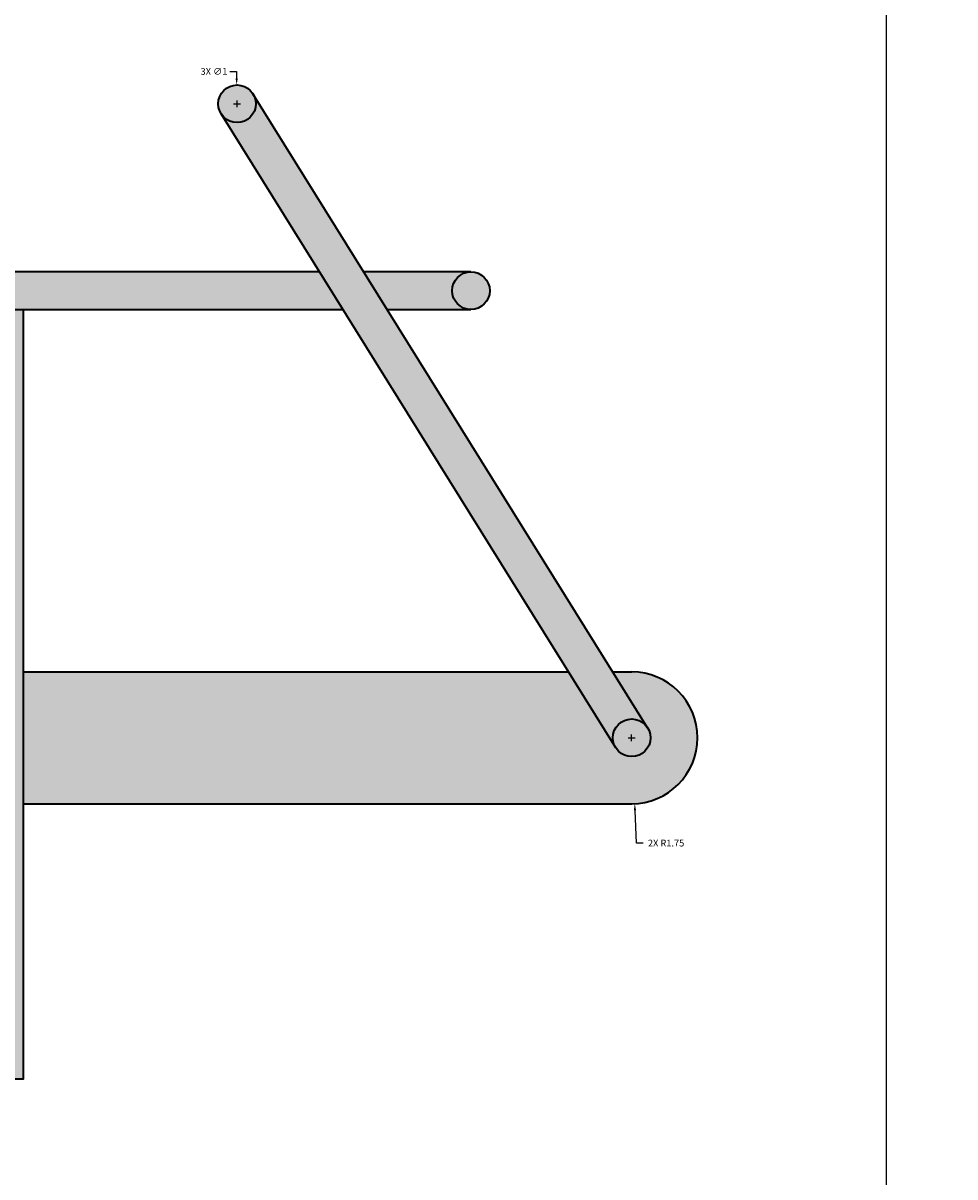
# Model space of a CAD drawing. Units: millimetres. Extents: x -11 to 280, y -4 to 208.
# Tile 54 of 55: x 237 to 262, y 142 to 173. Entities that reach past the tile are written whole.
import ezdxf

# ---------------------------------------------------------------- set-up
doc = ezdxf.new("R2010")
doc.units = ezdxf.units.MM
for name, color, linetype, lineweight in [('M-DIMS', 2, 'Continuous', 18), ('M-HYDR-EQPM', 7, 'Continuous', 35), ('M-HYDR-EQPM-PATT', 252, 'Continuous', 13)]:
    doc.layers.add(name, color=color, linetype=linetype, lineweight=lineweight)
doc.layers.add('M-HYDR-SUCT-PATT', color=221, linetype='Continuous', lineweight=13, true_color=0xff7fdf)
doc.styles.get("Standard").update_dxf_attribs({"font": 'arial.ttf'})
doc.dimstyles.get("Standard").update_dxf_attribs({"dimtxt": 0.18, "dimasz": 0.18, "dimexe": 0.18, "dimexo": 0.0625, "dimgap": 0.09, "dimtad": 0, "dimtih": 1, "dimtoh": 1, "dimdec": 4, "dimzin": 0, "dimdsep": 46, "dimtxsty": 'Standard', "dimcen": 0.09, "dimadec": 0, "dimazin": 0, "dimtfac": 1, "dimtdec": 4, "dimtofl": 0, "dimtmove": 0, "dimatfit": 3, "dimfxl": 1, "dimtolj": 1, "dimtzin": 0, "dimarcsym": 0})

# ---------------------------------------------------------------- blocks, each defined once
blk = doc.blocks.new('*D5')
at = {"layer": 'Defpoints', "color": 0, "transparency": 16777216}
for p in [(24.759, 192.645), (-10.087, 11.435), (261.686, 11.435)]:
    blk.add_point(p, dxfattribs=at)
at = {"layer": 'M-DIMS', "color": 0, "lineweight": -2, "transparency": 16777216}
for p, q in [((24.696, 192.645), (-10.267, 192.645)), ((-10.087, 192.465), (-10.087, 102.222)), ((-10.087, 11.615), (-10.087, 101.858)), ((261.624, 11.435), (-10.267, 11.435))]:
    blk.add_line(p, q, dxfattribs=at)
at = {"layer": 'M-DIMS', "color": 0, "transparency": 16777216}
for points in [[(-10.117, 192.465), (-10.057, 192.465), (-10.087, 192.645)], [(-10.117, 11.615), (-10.057, 11.615), (-10.087, 11.435)]]:
    blk.add_solid(points, dxfattribs=at)
at = {"layer": 'M-DIMS', "color": 0, "transparency": 16777216, "insert": (-10.087, 102.04), "char_height": 0.18, "attachment_point": 5}
blk.add_mtext('\\A1;181.2', dxfattribs=at)
blk = doc.blocks.new('*D22')
at = {"layer": 'Defpoints', "color": 0, "transparency": 16777216}
for p in [(259.871, 207.495), (231.68, 34.723), (259.871, 34.723)]:
    blk.add_point(p, dxfattribs=at)
at = {"layer": 'M-DIMS', "color": 0, "lineweight": -2, "transparency": 16777216}
for p, q in [((231.68, 34.785), (231.68, 207.675)), ((231.86, 207.495), (245.38, 207.495)), ((259.691, 207.495), (246.171, 207.495)), ((259.871, 34.785), (259.871, 207.675))]:
    blk.add_line(p, q, dxfattribs=at)
at = {"layer": 'M-DIMS', "color": 0, "transparency": 16777216}
for points in [[(231.86, 207.525), (231.86, 207.465), (231.68, 207.495)], [(259.691, 207.525), (259.691, 207.465), (259.871, 207.495)]]:
    blk.add_solid(points, dxfattribs=at)
at = {"layer": 'M-DIMS', "color": 0, "transparency": 16777216, "insert": (245.776, 207.495), "char_height": 0.18, "attachment_point": 5}
blk.add_mtext('\\A1;28.19', dxfattribs=at)
blk = doc.blocks.new('*D33')
at = {"layer": 'Defpoints', "color": 0, "transparency": 16777216}
for p in [(242.61, 171.067), (242.625, 170.067)]:
    blk.add_point(p, dxfattribs=at)
at = {"layer": 'M-DIMS', "color": 0, "lineweight": -2, "transparency": 16777216}
for p, q in [((242.425, 171.427), (242.605, 171.427)), ((242.605, 171.427), (242.608, 171.247)), ((242.528, 170.567), (242.708, 170.567)), ((242.618, 170.477), (242.618, 170.657))]:
    blk.add_line(p, q, dxfattribs=at)
at = {"layer": 'M-DIMS', "color": 0, "transparency": 16777216}
blk.add_solid([(242.638, 171.247), (242.578, 171.246), (242.61, 171.067)], dxfattribs=at)
at = {"layer": 'M-DIMS', "color": 0, "transparency": 16777216, "insert": (242.007, 171.427), "char_height": 0.18, "attachment_point": 5}
blk.add_mtext('\\A1;3X ∅1', dxfattribs=at)
blk = doc.blocks.new('*D34')
at = {"layer": 'Defpoints', "color": 0, "transparency": 16777216}
for p in [(253.1, 153.727), (253.181, 151.979)]:
    blk.add_point(p, dxfattribs=at)
at = {"layer": 'M-DIMS', "color": 0, "lineweight": -2, "transparency": 16777216}
for p, q in [((253.01, 153.727), (253.19, 153.727)), ((253.1, 153.637), (253.1, 153.817)), ((253.229, 150.93), (253.189, 151.799)), ((253.409, 150.93), (253.229, 150.93))]:
    blk.add_line(p, q, dxfattribs=at)
at = {"layer": 'M-DIMS', "color": 0, "transparency": 16777216}
blk.add_solid([(253.219, 151.8), (253.159, 151.797), (253.181, 151.979)], dxfattribs=at)
at = {"layer": 'M-DIMS', "color": 0, "transparency": 16777216, "insert": (254.015, 150.93), "char_height": 0.18, "attachment_point": 5}
blk.add_mtext('\\A1;2X R1.75', dxfattribs=at)

msp = doc.modelspace()

# ---------------------------------------------------------------- hatches: boundary and pattern name
at = {"layer": 'M-HYDR-EQPM-PATT'}
h = msp.add_hatch(color=256, dxfattribs=at)
h.set_gradient(color1=(0, 255, 255), color2=(34, 52, 110), tint=1, name='INVCYLINDER')
h.paths.add_polyline_path([(243.0423, 170.8308, -0.1401047), (243.1178, 170.5666, -0.7542249), (242.1933, 170.3024), (252.676, 153.4626, -0.1401047), (252.6005, 153.7268, -0.7542249), (253.5249, 153.991)])
h.paths.add_polyline_path([(243.1178, 170.5666, 0.1401047), (243.0423, 170.8308, 0.7542249), (242.1178, 170.5666, 1)])
h.paths.add_polyline_path([(252.6005, 153.7268, 0.1401047), (252.676, 153.4626, 0.7542249), (253.6005, 153.7268, 1)])
h = msp.add_hatch(color=256, dxfattribs=at)
h.set_gradient(color1=(248, 153, 30), color2=(248, 153, 30), tint=1)
h.paths.add_polyline_path([(236.9353, 165.103), (205.5315, 165.103), (205.5315, 144.6609), (236.9353, 144.6609)])
h.paths.add_polyline_path([(244.8074, 166.103), (205.5315, 166.103), (205.5315, 165.103), (236.9353, 165.103), (245.4299, 165.103)])
h.paths.add_polyline_path([(248.3313, 165.603, -0.4142136), (248.8313, 166.103), (245.9853, 166.103), (246.6078, 165.103), (248.8313, 165.103, -0.4142136)])
h.paths.add_polyline_path([(249.3313, 165.603, 1), (248.3313, 165.603, 0.4142136), (248.8313, 165.103, 0.4142136)])
at = {"layer": 'M-HYDR-SUCT-PATT'}
h = msp.add_hatch(color=256, dxfattribs=at)
h.set_gradient(color1=(255, 127, 223), color2=(255, 127, 223), tint=1, name='INVCYLINDER')
h.paths.add_polyline_path([(91.3629, 155.4768), (91.3629, 132.4768), (58.3629, 132.4768), (58.3629, 153.9768), (54.8629, 153.9768), (54.8629, 128.9768), (94.8629, 128.9768), (94.8629, 151.9768), (205.5315, 151.9768), (205.5315, 155.4768)])
h.paths.add_polyline_path([(91.3, 114.9452, 1), (78.8273, 114.9452), (78.8273, 108.8141), (42.6453, 108.8141), (42.6453, 153.9768), (39.1453, 153.9768), (39.1453, 105.3141), (78.8273, 105.3141), (78.8273, 98.1491, 1), (91.3, 98.1491), (91.3, 105.3141), (95.5776, 105.3141), (95.5776, 108.8141), (91.3, 108.8141)])
h.paths.add_polyline_path([(228.7, 138.4081), (232.2, 138.4081), (232.2, 144.6609), (228.7, 144.6609)])
h.paths.add_polyline_path([(253.1005, 151.9768, 1), (253.1005, 155.4768), (252.6001, 155.4768), (253.5249, 153.991, -0.1401047), (253.6005, 153.7268, -0.7542249), (252.676, 153.4626), (251.4221, 155.4768), (236.9353, 155.4768), (236.9353, 151.9768)])
h.paths.add_polyline_path([(30.8182, 40.7626), (30.8182, 36.7626), (60.8182, 36.7626), (60.8182, 40.7626)])

# ---------------------------------------------------------------- linework, layer by layer
at = {"layer": 'M-HYDR-EQPM'}
for p, q in [((253.5249, 153.991), (243.0423, 170.8308)), ((252.676, 153.4626), (242.1933, 170.3024)), ((244.8074, 166.103), (205.5315, 166.103)), ((248.8313, 166.103), (245.9853, 166.103)), ((236.9353, 165.103), (245.4299, 165.103)), ((246.6078, 165.103), (248.8313, 165.103))]:
    msp.add_line(p, q, dxfattribs=at)
msp.add_lwpolyline([(205.5315, 165.103), (236.9353, 165.103), (236.9353, 144.6609), (205.5315, 144.6609)], close=True, dxfattribs=at)
for points in [[(236.9353, 155.4768), (251.4221, 155.4768)], [(252.6001, 155.4768), (253.1005, 155.4768)], [(236.9353, 151.9768), (253.1005, 151.9768)]]:
    msp.add_lwpolyline(points, dxfattribs=at)
for centre in [(242.6178, 170.5666), (248.8313, 165.603), (253.1005, 153.7268)]:
    msp.add_circle(centre, 0.5, dxfattribs=at)
msp.add_arc((253.1005, 153.7268), 1.75, 270, 90, dxfattribs=at)

# ---------------------------------------------------------------- dimensions: what is measured, and where the dimension line sits
at = {"layer": 'M-DIMS'}
dim = msp.add_linear_dim(base=(259.871, 207.495), p1=(231.6803, 34.7226), p2=(259.871, 34.7226), dimstyle='Standard', override={"dimdec": 2, "dimlfac": 1, "dimrnd": 0, "dimzin": 0, "dimdsep": 46, "dimlunit": 2}, dxfattribs=at)
dim.commit()
dim.dimension.update_dxf_attribs({"geometry": '*D22', "text_midpoint": (245.7757, 207.495)})
dim = msp.add_linear_dim(base=(-10.0865, 11.4346), p1=(24.7588, 192.645), p2=(261.6863, 11.4346), angle=90, dimstyle='Standard', override={"dimdec": 1, "dimlfac": 1, "dimrnd": 0, "dimzin": 0, "dimdsep": 46, "dimlunit": 2}, dxfattribs=at)
dim.commit()
dim.dimension.update_dxf_attribs({"geometry": '*D5', "text_midpoint": (-10.0865, 102.0398)})
dim = msp.add_diameter_dim_2p(p1=(242.6251, 170.0666), p2=(242.6105, 171.0665), text='3X <>', dimstyle='Standard', override={"dimdec": 0, "dimlfac": 1, "dimrnd": 0, "dimzin": 0, "dimdsep": 46, "dimlunit": 2}, dxfattribs=at)
dim.commit()
dim.dimension.update_dxf_attribs({"geometry": '*D33', "text_midpoint": (242.0071, 171.4265), "dimtype": 163})
dim = msp.add_radius_dim(center=(253.1005, 153.7268), mpoint=(253.181, 151.9787), text='2X <>', dimstyle='Standard', override={"dimdec": 2, "dimlfac": 1, "dimrnd": 0, "dimzin": 0, "dimdsep": 46, "dimlunit": 2}, dxfattribs=at)
dim.commit()
dim.dimension.update_dxf_attribs({"geometry": '*D34', "text_midpoint": (254.0148, 150.9298), "dimtype": 164})

doc.saveas('drawing.dxf')
